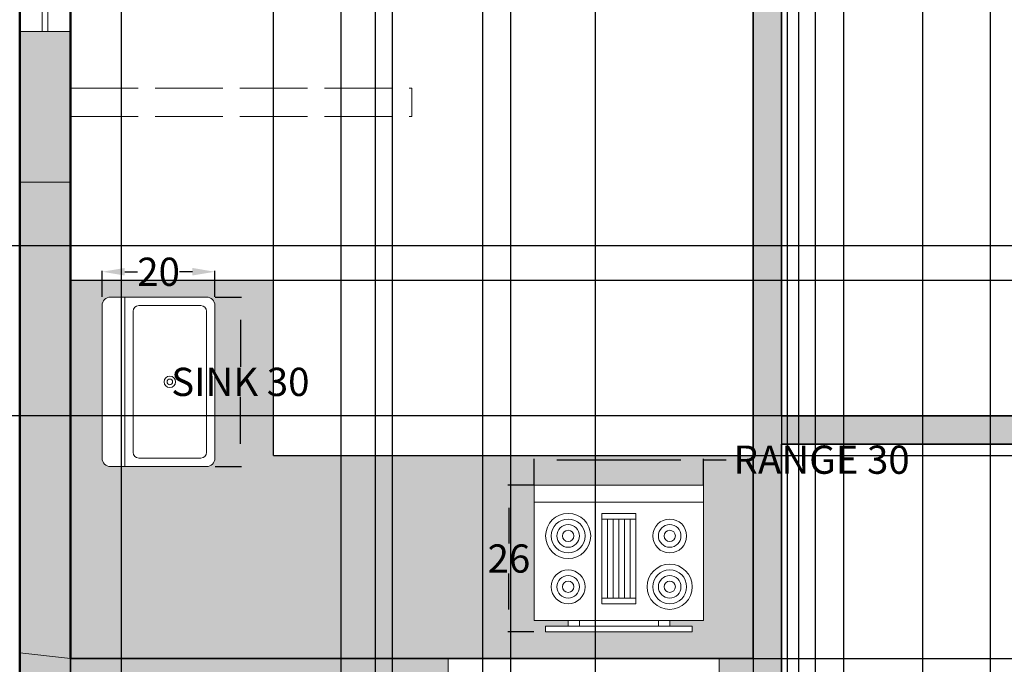
# Model space of a CAD drawing. Units: inches. Extents: x 882 to 1363, y 890 to 1847.
# Tile 3 of 9: x 983 to 1157, y 1106 to 1220. Entities that reach past the tile are written whole.
import ezdxf

# ---------------------------------------------------------------- set-up
doc = ezdxf.new("R2010")
doc.units = ezdxf.units.IN
doc.header["$MEASUREMENT"] = 0
doc.linetypes.add('ACAD_ISO02W100', pattern=[15, 12, -3])
for name, color, linetype, lineweight in [('A-ANNO-DIMS', 2, 'Continuous', 18), ('A-EQPM', 8, 'Continuous', 18), ('A-FLOR-CASE', 7, 'Continuous', 25), ('A-WALL-OVHD', 7, 'ACAD_ISO02W100', 18), ('A-WALL-PATT-BNDY', 7, 'Continuous', 13), ('inner wall', 50, 'Continuous', 35), ('outer wall', 40, 'Continuous', 50), ('sanitary', 231, 'Continuous', 18), ('windows', 226, 'Continuous', 18)]:
    doc.layers.add(name, color=color, linetype=linetype, lineweight=lineweight)
doc.layers.add('A-FLOR-CASE-PATT', color=15, linetype='Continuous', lineweight=13, true_color=0x9c4f2b)
doc.layers.add('A-WALL-PATT', color=251, linetype='Continuous', lineweight=13, true_color=0x636466)
doc.styles.get("Standard").update_dxf_attribs({"font": 'arial.ttf'})
doc.dimstyles.get("Standard").update_dxf_attribs({"dimtxt": 5, "dimasz": 4, "dimexe": 0.18, "dimexo": 0.0625, "dimgap": 0.09, "dimtad": 0, "dimtih": 1, "dimtoh": 1, "dimdec": 1, "dimzin": 0, "dimdsep": 46, "dimlunit": 3, "dimtxsty": 'Standard', "dimcen": 0.09, "dimadec": 0, "dimazin": 0, "dimtfac": 1, "dimtdec": 1, "dimtofl": 0, "dimtmove": 0, "dimatfit": 3, "dimfxl": 1, "dimtolj": 1, "dimtzin": 0, "dimarcsym": 0})

# ---------------------------------------------------------------- blocks, each defined once
blk = doc.blocks.new('Range-Oven - 30 in top')
for p, q in [((0, -3), (30, -3)), ((12, -6), (18, -6)), ((13, -20), (13, -6)), ((14, -6), (14, -20)), ((15, -20), (15, -6)), ((16, -6), (16, -20)), ((17, -20), (17, -6)), ((18, -20), (12, -20)), ((6, -24), (6, -25)), ((8, -25), (8, -24)), ((22, -25), (22, -24)), ((24, -24), (24, -25))]:
    blk.add_line(p, q)
for points in [[(0, -24), (0, 0), (30, 0), (30, -24)], [(12, -21), (12, -5), (18, -5), (18, -21)], [(2, -26), (2, -25), (28, -25), (28, -26)]]:
    blk.add_lwpolyline(points, close=True)
for centre, radius in [((6, -9), 4), ((6, -9), 3), ((24, -9), 3), ((6, -9), 2), ((6, -9), 1), ((24, -9), 2), ((24, -9), 1), ((6, -18), 3), ((24, -18), 4), ((24, -18), 3), ((6, -18), 2), ((6, -18), 1), ((24, -18), 2), ((24, -18), 1)]:
    blk.add_circle(centre, radius)
blk = doc.blocks.new('Sink-single - 30 in top')
blk.add_line((-15, -3.999996), (15, -3.999996))
for points in [[(-13.5, 0), (13.5, 0)], [(-15, -18.499996), (-15, -1.5)], [(15, -1.5), (15, -18.499996)], [(-13.5, -17.499996), (-13.5, -6.499996)], [(-12.5, -5.499996), (12.5, -5.499996)], [(13.5, -6.499996), (13.5, -17.499996)], [(12.5, -18.499996), (-12.5, -18.499996)], [(13.5, -19.999996), (-13.5, -19.999996)]]:
    blk.add_lwpolyline(points)
for radius in [1, 0.5]:
    blk.add_circle((0, -11.999996), radius)
for centre, radius, start, end in [((-13.5, -1.5), 1.5, 90, 180), ((13.5, -1.5), 1.5, 0, 90), ((-12.5, -6.499996), 1, 90, 180), ((12.5, -6.499996), 1, 0, 90), ((-13.5, -18.499996), 1.5, 180, 270), ((-12.5, -17.499996), 1, 180, 270), ((12.5, -17.499996), 1, 270, 0), ((13.5, -18.499996), 1.5, 270, 0)]:
    blk.add_arc(centre, radius, start, end)
blk = doc.blocks.new('WIN-48IN-9IN')
for p, q in [((4, 0), (4, 48)), ((5, 0), (5, 48))]:
    blk.add_line(p, q)
blk.add_lwpolyline([(0, 48), (9, 48), (9, 0), (0, 0)], close=True)
blk = doc.blocks.new('*D29')
at = {"layer": 'A-ANNO-DIMS', "color": 0, "lineweight": -2, "transparency": 16777216}
for p, q in [((1074.04, 1137.54), (1074.04, 1142.16)), ((1078.04, 1141.98), (1100.04, 1141.98)), ((1104.04, 1137.54), (1104.04, 1142.16)), ((1104.04, 1141.98), (1108.04, 1141.98))]:
    blk.add_line(p, q, dxfattribs=at)
at = {"layer": 'A-ANNO-DIMS', "color": 0, "transparency": 16777216}
for points in [[(1078.04, 1142.64), (1078.04, 1141.31), (1074.04, 1141.98)], [(1100.04, 1142.64), (1100.04, 1141.31), (1104.04, 1141.98)]]:
    blk.add_solid(points, dxfattribs=at)
at = {"layer": 'Defpoints', "color": 0, "transparency": 16777216}
for p in [(1104.04, 1141.98), (1074.04, 1137.48), (1104.04, 1137.48)]:
    blk.add_point(p, dxfattribs=at)
at = {"layer": 'A-ANNO-DIMS', "color": 0, "transparency": 16777216, "insert": (1124.96, 1141.98), "char_height": 5, "attachment_point": 5}
blk.add_mtext('\\A1;RANGE 30', dxfattribs=at)
blk = doc.blocks.new('*D30')
at = {"layer": 'A-ANNO-DIMS', "color": 0, "lineweight": -2, "transparency": 16777216}
for p, q in [((1073.98, 1137.48), (1069.36, 1137.48)), ((1069.54, 1133.48), (1069.54, 1127.12)), ((1069.54, 1115.48), (1069.54, 1121.83)), ((1073.98, 1111.48), (1069.36, 1111.48))]:
    blk.add_line(p, q, dxfattribs=at)
at = {"layer": 'A-ANNO-DIMS', "color": 0, "transparency": 16777216}
for points in [[(1068.87, 1133.48), (1070.2, 1133.48), (1069.54, 1137.48)], [(1068.87, 1115.48), (1070.2, 1115.48), (1069.54, 1111.48)]]:
    blk.add_solid(points, dxfattribs=at)
at = {"layer": 'Defpoints', "color": 0, "transparency": 16777216}
for p in [(1069.54, 1137.48), (1074.04, 1137.48), (1074.04, 1111.48)]:
    blk.add_point(p, dxfattribs=at)
at = {"layer": 'A-ANNO-DIMS', "color": 0, "transparency": 16777216, "insert": (1069.54, 1124.48), "char_height": 5, "attachment_point": 5}
blk.add_mtext('\\A1;26', dxfattribs=at)
blk = doc.blocks.new('*D31')
at = {"layer": 'A-ANNO-DIMS', "color": 0, "lineweight": -2, "transparency": 16777216}
for p, q in [((1017.51, 1170.76), (1022.13, 1170.76)), ((1021.95, 1166.76), (1021.95, 1158.44)), ((1021.95, 1144.76), (1021.95, 1153.09)), ((1017.51, 1140.76), (1022.13, 1140.76))]:
    blk.add_line(p, q, dxfattribs=at)
at = {"layer": 'A-ANNO-DIMS', "color": 0, "transparency": 16777216}
for points in [[(1021.28, 1166.76), (1022.61, 1166.76), (1021.95, 1170.76)], [(1021.28, 1144.76), (1022.61, 1144.76), (1021.95, 1140.76)]]:
    blk.add_solid(points, dxfattribs=at)
at = {"layer": 'Defpoints', "color": 0, "transparency": 16777216}
for p in [(1017.45, 1170.76), (1021.95, 1170.76), (1017.45, 1140.76)]:
    blk.add_point(p, dxfattribs=at)
at = {"layer": 'A-ANNO-DIMS', "color": 0, "transparency": 16777216, "insert": (1021.95, 1155.76), "char_height": 5, "attachment_point": 5}
blk.add_mtext('\\A1;SINK 30', dxfattribs=at)
blk = doc.blocks.new('*D32')
at = {"layer": 'A-ANNO-DIMS', "color": 0, "lineweight": -2, "transparency": 16777216}
for p, q in [((997.45, 1170.83), (997.45, 1175.44)), ((1001.45, 1175.26), (1003.74, 1175.26)), ((1013.45, 1175.26), (1011.15, 1175.26)), ((1017.45, 1170.83), (1017.45, 1175.44))]:
    blk.add_line(p, q, dxfattribs=at)
at = {"layer": 'A-ANNO-DIMS', "color": 0, "transparency": 16777216}
for points in [[(1001.45, 1175.93), (1001.45, 1174.6), (997.45, 1175.26)], [(1013.45, 1175.93), (1013.45, 1174.6), (1017.45, 1175.26)]]:
    blk.add_solid(points, dxfattribs=at)
at = {"layer": 'Defpoints', "color": 0, "transparency": 16777216}
for p in [(997.45, 1175.26), (997.45, 1170.76), (1017.45, 1170.76)]:
    blk.add_point(p, dxfattribs=at)
at = {"layer": 'A-ANNO-DIMS', "color": 0, "transparency": 16777216, "insert": (1007.45, 1175.26), "char_height": 5, "attachment_point": 5}
blk.add_mtext('\\A1;20', dxfattribs=at)
blk = doc.blocks.new('*D40')
at = {"layer": 'A-ANNO-DIMS', "color": 0, "lineweight": -2, "transparency": 16777216}
for p, q in [((991.84, 1758.69), (991.84, 893.37)), ((1064.84, 1758.69), (1064.84, 893.37)), ((995.84, 893.55), (1024.69, 893.55)), ((1060.84, 893.55), (1031.99, 893.55))]:
    blk.add_line(p, q, dxfattribs=at)
at = {"layer": 'A-ANNO-DIMS', "color": 0, "transparency": 16777216}
for points in [[(995.84, 894.21), (995.84, 892.88), (991.84, 893.55)], [(1060.84, 894.21), (1060.84, 892.88), (1064.84, 893.55)]]:
    blk.add_solid(points, dxfattribs=at)
at = {"layer": 'Defpoints', "color": 0, "transparency": 16777216}
for p in [(991.84, 1758.75), (1064.84, 1758.75), (1064.84, 893.55)]:
    blk.add_point(p, dxfattribs=at)
at = {"layer": 'A-ANNO-DIMS', "color": 0, "transparency": 16777216, "insert": (1028.34, 893.55), "char_height": 5, "attachment_point": 5}
blk.add_mtext('\\A1;73', dxfattribs=at)
blk = doc.blocks.new('*D41')
at = {"layer": 'A-ANNO-DIMS', "color": 0, "lineweight": -2, "transparency": 16777216}
for p, q in [((1069.84, 1758.69), (1069.84, 893.37)), ((1154.84, 1758.69), (1154.84, 893.37)), ((1073.84, 893.55), (1108.65, 893.55)), ((1150.84, 893.55), (1116.03, 893.55))]:
    blk.add_line(p, q, dxfattribs=at)
at = {"layer": 'A-ANNO-DIMS', "color": 0, "transparency": 16777216}
for points in [[(1073.84, 894.21), (1073.84, 892.88), (1069.84, 893.55)], [(1150.84, 894.21), (1150.84, 892.88), (1154.84, 893.55)]]:
    blk.add_solid(points, dxfattribs=at)
at = {"layer": 'Defpoints', "color": 0, "transparency": 16777216}
for p in [(1069.84, 1758.75), (1154.84, 1758.75), (1154.84, 893.55)]:
    blk.add_point(p, dxfattribs=at)
at = {"layer": 'A-ANNO-DIMS', "color": 0, "transparency": 16777216, "insert": (1112.34, 893.55), "char_height": 5, "attachment_point": 5}
blk.add_mtext('\\A1;85', dxfattribs=at)
blk = doc.blocks.new('*D47')
at = {"layer": 'A-ANNO-DIMS', "color": 0, "lineweight": -2, "transparency": 16777216}
for p, q in [((1123.84, 1567.69), (1123.84, 893.37)), ((1128.84, 1567.69), (1128.84, 893.37)), ((1119.84, 893.55), (1115.84, 893.55)), ((1132.84, 893.55), (1136.84, 893.55))]:
    blk.add_line(p, q, dxfattribs=at)
at = {"layer": 'A-ANNO-DIMS', "color": 0, "transparency": 16777216}
for points in [[(1119.84, 894.21), (1119.84, 892.88), (1123.84, 893.55)], [(1132.84, 894.21), (1132.84, 892.88), (1128.84, 893.55)]]:
    blk.add_solid(points, dxfattribs=at)
at = {"layer": 'Defpoints', "color": 0, "transparency": 16777216}
for p in [(1123.84, 1567.75), (1128.84, 1567.75), (1128.84, 893.55)]:
    blk.add_point(p, dxfattribs=at)
at = {"layer": 'A-ANNO-DIMS', "color": 0, "transparency": 16777216, "insert": (1126.34, 893.55), "char_height": 5, "attachment_point": 5}
blk.add_mtext('\\A1;5', dxfattribs=at)
blk = doc.blocks.new('*D48')
at = {"layer": 'A-ANNO-DIMS', "color": 0, "lineweight": -2, "transparency": 16777216}
for p, q in [((1084.84, 1562.69), (1084.84, 893.37)), ((1120.84, 1562.69), (1120.84, 893.37)), ((1088.84, 893.55), (1099.17, 893.55)), ((1116.84, 893.55), (1106.51, 893.55))]:
    blk.add_line(p, q, dxfattribs=at)
at = {"layer": 'A-ANNO-DIMS', "color": 0, "transparency": 16777216}
for points in [[(1088.84, 894.21), (1088.84, 892.88), (1084.84, 893.55)], [(1116.84, 894.21), (1116.84, 892.88), (1120.84, 893.55)]]:
    blk.add_solid(points, dxfattribs=at)
at = {"layer": 'Defpoints', "color": 0, "transparency": 16777216}
for p in [(1084.84, 1562.75), (1120.84, 1562.75), (1120.84, 893.55)]:
    blk.add_point(p, dxfattribs=at)
at = {"layer": 'A-ANNO-DIMS', "color": 0, "transparency": 16777216, "insert": (1102.84, 893.55), "char_height": 5, "attachment_point": 5}
blk.add_mtext('\\A1;36', dxfattribs=at)
blk = doc.blocks.new('*D51')
at = {"layer": 'A-ANNO-DIMS', "color": 0, "lineweight": -2, "transparency": 16777216}
for p, q in [((982.84, 1767.69), (982.84, 893.37)), ((1000.84, 1767.69), (1000.84, 893.37)), ((986.84, 893.55), (996.84, 893.55)), ((1000.84, 893.55), (1004.84, 893.55))]:
    blk.add_line(p, q, dxfattribs=at)
at = {"layer": 'A-ANNO-DIMS', "color": 0, "transparency": 16777216}
for points in [[(986.84, 894.21), (986.84, 892.88), (982.84, 893.55)], [(996.84, 894.21), (996.84, 892.88), (1000.84, 893.55)]]:
    blk.add_solid(points, dxfattribs=at)
at = {"layer": 'Defpoints', "color": 0, "transparency": 16777216}
for p in [(982.84, 1767.75), (1000.84, 1767.75), (1000.84, 893.55)]:
    blk.add_point(p, dxfattribs=at)
at = {"layer": 'A-ANNO-DIMS', "color": 0, "transparency": 16777216, "insert": (1015.08, 893.55), "char_height": 5, "attachment_point": 5}
blk.add_mtext('\\A1;18.006', dxfattribs=at)
blk = doc.blocks.new('*D52')
at = {"layer": 'A-ANNO-DIMS', "color": 0, "lineweight": -2, "transparency": 16777216}
for p, q in [((1048.84, 1767.69), (1048.84, 893.37)), ((1118.86, 1767.69), (1118.86, 893.37)), ((1052.84, 893.55), (1075.83, 893.55)), ((1114.86, 893.55), (1091.87, 893.55))]:
    blk.add_line(p, q, dxfattribs=at)
at = {"layer": 'A-ANNO-DIMS', "color": 0, "transparency": 16777216}
for points in [[(1052.84, 894.21), (1052.84, 892.88), (1048.84, 893.55)], [(1114.86, 894.21), (1114.86, 892.88), (1118.86, 893.55)]]:
    blk.add_solid(points, dxfattribs=at)
at = {"layer": 'Defpoints', "color": 0, "transparency": 16777216}
for p in [(1048.84, 1767.75), (1118.86, 1767.75), (1118.86, 893.55)]:
    blk.add_point(p, dxfattribs=at)
at = {"layer": 'A-ANNO-DIMS', "color": 0, "transparency": 16777216, "insert": (1083.85, 893.55), "char_height": 5, "attachment_point": 5}
blk.add_mtext('\\A1;70.01', dxfattribs=at)
blk = doc.blocks.new('*D53')
at = {"layer": 'A-ANNO-DIMS', "color": 0, "lineweight": -2, "transparency": 16777216}
for p, q in [((1142.86, 1767.69), (1142.86, 893.37)), ((1171.41, 1767.69), (1171.41, 893.37)), ((1138.86, 893.55), (1134.86, 893.55)), ((1175.41, 893.55), (1179.41, 893.55))]:
    blk.add_line(p, q, dxfattribs=at)
at = {"layer": 'A-ANNO-DIMS', "color": 0, "transparency": 16777216}
for points in [[(1138.86, 894.21), (1138.86, 892.88), (1142.86, 893.55)], [(1175.41, 894.21), (1175.41, 892.88), (1171.41, 893.55)]]:
    blk.add_solid(points, dxfattribs=at)
at = {"layer": 'Defpoints', "color": 0, "transparency": 16777216}
for p in [(1142.86, 1767.75), (1171.41, 1767.75), (1171.41, 893.55)]:
    blk.add_point(p, dxfattribs=at)
at = {"layer": 'A-ANNO-DIMS', "color": 0, "transparency": 16777216, "insert": (1157.14, 893.55), "char_height": 5, "attachment_point": 5}
blk.add_mtext('\\A1;28.554', dxfattribs=at)
blk = doc.blocks.new('*D61')
at = {"layer": 'A-ANNO-DIMS', "color": 0, "lineweight": -2, "transparency": 16777216}
for p, q in [((991.84, 1348.69), (991.84, 893.37)), ((1128.84, 1348.69), (1128.84, 893.37)), ((995.84, 893.55), (1054.96, 893.55)), ((1124.84, 893.55), (1065.72, 893.55))]:
    blk.add_line(p, q, dxfattribs=at)
at = {"layer": 'A-ANNO-DIMS', "color": 0, "transparency": 16777216}
for points in [[(995.84, 894.21), (995.84, 892.88), (991.84, 893.55)], [(1124.84, 894.21), (1124.84, 892.88), (1128.84, 893.55)]]:
    blk.add_solid(points, dxfattribs=at)
at = {"layer": 'Defpoints', "color": 0, "transparency": 16777216}
for p in [(991.84, 1348.75), (1128.84, 1348.75), (1128.84, 893.55)]:
    blk.add_point(p, dxfattribs=at)
at = {"layer": 'A-ANNO-DIMS', "color": 0, "transparency": 16777216, "insert": (1060.34, 893.55), "char_height": 5, "attachment_point": 5}
blk.add_mtext('\\A1;137', dxfattribs=at)
blk = doc.blocks.new('*D62')
at = {"layer": 'A-ANNO-DIMS', "color": 0, "lineweight": -2, "transparency": 16777216}
for p, q in [((991.9, 1348.75), (1353.22, 1348.75)), ((1353.04, 1344.75), (1353.04, 1230.35)), ((1353.04, 1110.75), (1353.04, 1225.15)), ((991.9, 1106.75), (1353.22, 1106.75))]:
    blk.add_line(p, q, dxfattribs=at)
at = {"layer": 'A-ANNO-DIMS', "color": 0, "transparency": 16777216}
for points in [[(1352.38, 1344.75), (1353.71, 1344.75), (1353.04, 1348.75)], [(1352.38, 1110.75), (1353.71, 1110.75), (1353.04, 1106.75)]]:
    blk.add_solid(points, dxfattribs=at)
at = {"layer": 'Defpoints', "color": 0, "transparency": 16777216}
for p in [(991.84, 1348.75), (991.84, 1106.75), (1353.04, 1106.75)]:
    blk.add_point(p, dxfattribs=at)
at = {"layer": 'A-ANNO-DIMS', "color": 0, "transparency": 16777216, "insert": (1353.04, 1227.75), "char_height": 5, "attachment_point": 5}
blk.add_mtext('\\A1;242', dxfattribs=at)
blk = doc.blocks.new('*D63')
at = {"layer": 'A-ANNO-DIMS', "color": 0, "lineweight": -2, "transparency": 16777216}
for p, q in [((991.84, 1106.69), (991.84, 893.37)), ((1112.84, 1106.69), (1112.84, 893.37)), ((995.84, 893.55), (1047.44, 893.55)), ((1108.84, 893.55), (1057.23, 893.55))]:
    blk.add_line(p, q, dxfattribs=at)
at = {"layer": 'A-ANNO-DIMS', "color": 0, "transparency": 16777216}
for points in [[(995.84, 894.21), (995.84, 892.88), (991.84, 893.55)], [(1108.84, 894.21), (1108.84, 892.88), (1112.84, 893.55)]]:
    blk.add_solid(points, dxfattribs=at)
at = {"layer": 'Defpoints', "color": 0, "transparency": 16777216}
for p in [(991.84, 1106.75), (1112.84, 1106.75), (1112.84, 893.55)]:
    blk.add_point(p, dxfattribs=at)
at = {"layer": 'A-ANNO-DIMS', "color": 0, "transparency": 16777216, "insert": (1052.34, 893.55), "char_height": 5, "attachment_point": 5}
blk.add_mtext('\\A1;121', dxfattribs=at)
blk = doc.blocks.new('*D64')
at = {"layer": 'A-ANNO-DIMS', "color": 0, "lineweight": -2, "transparency": 16777216}
for p, q in [((1117.84, 1269.69), (1117.84, 893.37)), ((1243.84, 1269.69), (1243.84, 893.37)), ((1121.84, 893.55), (1175.46, 893.55)), ((1239.84, 893.55), (1186.22, 893.55))]:
    blk.add_line(p, q, dxfattribs=at)
at = {"layer": 'A-ANNO-DIMS', "color": 0, "transparency": 16777216}
for points in [[(1121.84, 894.21), (1121.84, 892.88), (1117.84, 893.55)], [(1239.84, 894.21), (1239.84, 892.88), (1243.84, 893.55)]]:
    blk.add_solid(points, dxfattribs=at)
at = {"layer": 'Defpoints', "color": 0, "transparency": 16777216}
for p in [(1117.84, 1269.75), (1243.84, 1269.75), (1243.84, 893.55)]:
    blk.add_point(p, dxfattribs=at)
at = {"layer": 'A-ANNO-DIMS', "color": 0, "transparency": 16777216, "insert": (1180.84, 893.55), "char_height": 5, "attachment_point": 5}
blk.add_mtext('\\A1;126', dxfattribs=at)
blk = doc.blocks.new('*D65')
at = {"layer": 'A-ANNO-DIMS', "color": 0, "lineweight": -2, "transparency": 16777216}
for p, q in [((1117.9, 1269.75), (1353.22, 1269.75)), ((1353.04, 1265.75), (1353.04, 1212.39)), ((1353.04, 1153.75), (1353.04, 1207.11)), ((1117.9, 1149.75), (1353.22, 1149.75))]:
    blk.add_line(p, q, dxfattribs=at)
at = {"layer": 'A-ANNO-DIMS', "color": 0, "transparency": 16777216}
for points in [[(1352.38, 1265.75), (1353.71, 1265.75), (1353.04, 1269.75)], [(1352.38, 1153.75), (1353.71, 1153.75), (1353.04, 1149.75)]]:
    blk.add_solid(points, dxfattribs=at)
at = {"layer": 'Defpoints', "color": 0, "transparency": 16777216}
for p in [(1117.84, 1269.75), (1353.04, 1269.75), (1117.84, 1149.75)]:
    blk.add_point(p, dxfattribs=at)
at = {"layer": 'A-ANNO-DIMS', "color": 0, "transparency": 16777216, "insert": (1353.04, 1209.75), "char_height": 5, "attachment_point": 5}
blk.add_mtext('\\A1;120', dxfattribs=at)
blk = doc.blocks.new('*D68')
at = {"layer": 'A-ANNO-DIMS', "color": 0, "lineweight": -2, "transparency": 16777216}
for p, q in [((1027.84, 1142.81), (1027.84, 1844.13)), ((1031.84, 1843.95), (1066.65, 1843.95)), ((1108.84, 1843.95), (1074.03, 1843.95)), ((1112.84, 1142.81), (1112.84, 1844.13))]:
    blk.add_line(p, q, dxfattribs=at)
at = {"layer": 'A-ANNO-DIMS', "color": 0, "transparency": 16777216}
for points in [[(1031.84, 1844.62), (1031.84, 1843.29), (1027.84, 1843.95)], [(1108.84, 1844.62), (1108.84, 1843.29), (1112.84, 1843.95)]]:
    blk.add_solid(points, dxfattribs=at)
at = {"layer": 'Defpoints', "color": 0, "transparency": 16777216}
for p in [(1112.84, 1843.95), (1027.84, 1142.75), (1112.84, 1142.75)]:
    blk.add_point(p, dxfattribs=at)
at = {"layer": 'A-ANNO-DIMS', "color": 0, "transparency": 16777216, "insert": (1070.34, 1843.95), "char_height": 5, "attachment_point": 5}
blk.add_mtext('\\A1;85', dxfattribs=at)
blk = doc.blocks.new('*D69')
at = {"layer": 'A-ANNO-DIMS', "color": 0, "lineweight": -2, "transparency": 16777216}
for p, q in [((1027.9, 1173.75), (1353.22, 1173.75)), ((1353.04, 1169.75), (1353.04, 1160.89)), ((1353.04, 1146.75), (1353.04, 1155.6)), ((1027.9, 1142.75), (1353.22, 1142.75))]:
    blk.add_line(p, q, dxfattribs=at)
at = {"layer": 'A-ANNO-DIMS', "color": 0, "transparency": 16777216}
for points in [[(1352.38, 1169.75), (1353.71, 1169.75), (1353.04, 1173.75)], [(1352.38, 1146.75), (1353.71, 1146.75), (1353.04, 1142.75)]]:
    blk.add_solid(points, dxfattribs=at)
at = {"layer": 'Defpoints', "color": 0, "transparency": 16777216}
for p in [(1027.84, 1173.75), (1353.04, 1173.75), (1027.84, 1142.75)]:
    blk.add_point(p, dxfattribs=at)
at = {"layer": 'A-ANNO-DIMS', "color": 0, "transparency": 16777216, "insert": (1353.04, 1158.25), "char_height": 5, "attachment_point": 5}
blk.add_mtext('\\A1;31', dxfattribs=at)
blk = doc.blocks.new('*D70')
at = {"layer": 'A-ANNO-DIMS', "color": 0, "lineweight": -2, "transparency": 16777216}
for p, q in [((1027.9, 1142.75), (1353.22, 1142.75)), ((1353.04, 1138.75), (1353.04, 1127.39)), ((1353.04, 1110.75), (1353.04, 1122.1)), ((991.9, 1106.75), (1353.22, 1106.75))]:
    blk.add_line(p, q, dxfattribs=at)
at = {"layer": 'A-ANNO-DIMS', "color": 0, "transparency": 16777216}
for points in [[(1352.38, 1138.75), (1353.71, 1138.75), (1353.04, 1142.75)], [(1352.38, 1110.75), (1353.71, 1110.75), (1353.04, 1106.75)]]:
    blk.add_solid(points, dxfattribs=at)
at = {"layer": 'Defpoints', "color": 0, "transparency": 16777216}
for p in [(1027.84, 1142.75), (991.84, 1106.75), (1353.04, 1106.75)]:
    blk.add_point(p, dxfattribs=at)
at = {"layer": 'A-ANNO-DIMS', "color": 0, "transparency": 16777216, "insert": (1353.04, 1124.75), "char_height": 5, "attachment_point": 5}
blk.add_mtext('\\A1;36', dxfattribs=at)
blk = doc.blocks.new('*D71')
at = {"layer": 'A-ANNO-DIMS', "color": 0, "lineweight": -2, "transparency": 16777216}
for p, q in [((1243.78, 1179.86), (906.46, 1179.86)), ((906.64, 1175.86), (906.64, 1167.45)), ((906.64, 1153.75), (906.64, 1162.16)), ((1243.78, 1149.75), (906.46, 1149.75))]:
    blk.add_line(p, q, dxfattribs=at)
at = {"layer": 'A-ANNO-DIMS', "color": 0, "transparency": 16777216}
for points in [[(905.97, 1175.86), (907.3, 1175.86), (906.64, 1179.86)], [(905.97, 1153.75), (907.3, 1153.75), (906.64, 1149.75)]]:
    blk.add_solid(points, dxfattribs=at)
at = {"layer": 'Defpoints', "color": 0, "transparency": 16777216}
for p in [(906.64, 1179.86), (1243.84, 1179.86), (1243.84, 1149.75)]:
    blk.add_point(p, dxfattribs=at)
at = {"layer": 'A-ANNO-DIMS', "color": 0, "transparency": 16777216, "insert": (906.64, 1164.8), "char_height": 5, "attachment_point": 5}
blk.add_mtext('\\A1;30.107', dxfattribs=at)
blk = doc.blocks.new('*D74')
at = {"layer": 'A-ANNO-DIMS', "color": 0, "lineweight": -2, "transparency": 16777216}
for p, q in [((991.84, 1002.81), (991.84, 1844.13)), ((995.84, 1843.95), (1012.06, 1843.95)), ((1035.84, 1843.95), (1019.62, 1843.95)), ((1039.84, 1002.81), (1039.84, 1844.13))]:
    blk.add_line(p, q, dxfattribs=at)
at = {"layer": 'A-ANNO-DIMS', "color": 0, "transparency": 16777216}
for points in [[(995.84, 1844.62), (995.84, 1843.29), (991.84, 1843.95)], [(1035.84, 1844.62), (1035.84, 1843.29), (1039.84, 1843.95)]]:
    blk.add_solid(points, dxfattribs=at)
at = {"layer": 'Defpoints', "color": 0, "transparency": 16777216}
for p in [(1039.84, 1843.95), (991.84, 1002.75), (1039.84, 1002.75)]:
    blk.add_point(p, dxfattribs=at)
at = {"layer": 'A-ANNO-DIMS', "color": 0, "transparency": 16777216, "insert": (1015.84, 1843.95), "char_height": 5, "attachment_point": 5}
blk.add_mtext('\\A1;48', dxfattribs=at)
blk = doc.blocks.new('*D77')
at = {"layer": 'A-ANNO-DIMS', "color": 0, "lineweight": -2, "transparency": 16777216}
for p, q in [((1117.9, 1144.75), (1353.22, 1144.75)), ((1353.04, 1140.75), (1353.04, 1125.89)), ((1353.04, 1105.75), (1353.04, 1120.6)), ((1117.9, 1101.75), (1353.22, 1101.75))]:
    blk.add_line(p, q, dxfattribs=at)
at = {"layer": 'A-ANNO-DIMS', "color": 0, "transparency": 16777216}
for points in [[(1352.38, 1140.75), (1353.71, 1140.75), (1353.04, 1144.75)], [(1352.38, 1105.75), (1353.71, 1105.75), (1353.04, 1101.75)]]:
    blk.add_solid(points, dxfattribs=at)
at = {"layer": 'Defpoints', "color": 0, "transparency": 16777216}
for p in [(1117.84, 1144.75), (1353.04, 1144.75), (1117.84, 1101.75)]:
    blk.add_point(p, dxfattribs=at)
at = {"layer": 'A-ANNO-DIMS', "color": 0, "transparency": 16777216, "insert": (1353.04, 1123.25), "char_height": 5, "attachment_point": 5}
blk.add_mtext('\\A1;43', dxfattribs=at)
blk = doc.blocks.new('*D85')
at = {"layer": 'A-ANNO-DIMS', "color": 0, "lineweight": -2, "transparency": 16777216}
for p, q in [((1045.84, 1562.69), (1045.84, 893.37)), ((1084.84, 1562.69), (1084.84, 893.37)), ((1049.84, 893.55), (1061.66, 893.55)), ((1080.84, 893.55), (1069.01, 893.55))]:
    blk.add_line(p, q, dxfattribs=at)
at = {"layer": 'A-ANNO-DIMS', "color": 0, "transparency": 16777216}
for points in [[(1049.84, 894.21), (1049.84, 892.88), (1045.84, 893.55)], [(1080.84, 894.21), (1080.84, 892.88), (1084.84, 893.55)]]:
    blk.add_solid(points, dxfattribs=at)
at = {"layer": 'Defpoints', "color": 0, "transparency": 16777216}
for p in [(1045.84, 1562.75), (1084.84, 1562.75), (1084.84, 893.55)]:
    blk.add_point(p, dxfattribs=at)
at = {"layer": 'A-ANNO-DIMS', "color": 0, "transparency": 16777216, "insert": (1065.34, 893.55), "char_height": 5, "attachment_point": 5}
blk.add_mtext('\\A1;39', dxfattribs=at)
blk = doc.blocks.new('*D88')
at = {"layer": 'A-ANNO-DIMS', "color": 0, "lineweight": -2, "transparency": 16777216}
for p, q in [((1128.84, 1567.69), (1128.84, 893.37)), ((1211.84, 1562.69), (1211.84, 893.37)), ((1132.84, 893.55), (1166.66, 893.55)), ((1207.84, 893.55), (1174.01, 893.55))]:
    blk.add_line(p, q, dxfattribs=at)
at = {"layer": 'A-ANNO-DIMS', "color": 0, "transparency": 16777216}
for points in [[(1132.84, 894.21), (1132.84, 892.88), (1128.84, 893.55)], [(1207.84, 894.21), (1207.84, 892.88), (1211.84, 893.55)]]:
    blk.add_solid(points, dxfattribs=at)
at = {"layer": 'Defpoints', "color": 0, "transparency": 16777216}
for p in [(1128.84, 1567.75), (1211.84, 1562.75), (1211.84, 893.55)]:
    blk.add_point(p, dxfattribs=at)
at = {"layer": 'A-ANNO-DIMS', "color": 0, "transparency": 16777216, "insert": (1170.34, 893.55), "char_height": 5, "attachment_point": 5}
blk.add_mtext('\\A1;83', dxfattribs=at)
blk = doc.blocks.new('*D89')
at = {"layer": 'A-ANNO-DIMS', "color": 0, "lineweight": -2, "transparency": 16777216}
for p, q in [((991.84, 1473.69), (991.84, 893.37)), ((1084.84, 1473.69), (1084.84, 893.37)), ((995.84, 893.55), (1034.67, 893.55)), ((1080.84, 893.55), (1042.01, 893.55))]:
    blk.add_line(p, q, dxfattribs=at)
at = {"layer": 'A-ANNO-DIMS', "color": 0, "transparency": 16777216}
for points in [[(995.84, 894.21), (995.84, 892.88), (991.84, 893.55)], [(1080.84, 894.21), (1080.84, 892.88), (1084.84, 893.55)]]:
    blk.add_solid(points, dxfattribs=at)
at = {"layer": 'Defpoints', "color": 0, "transparency": 16777216}
for p in [(991.84, 1473.75), (1084.84, 1473.75), (1084.84, 893.55)]:
    blk.add_point(p, dxfattribs=at)
at = {"layer": 'A-ANNO-DIMS', "color": 0, "transparency": 16777216, "insert": (1038.34, 893.55), "char_height": 5, "attachment_point": 5}
blk.add_mtext('\\A1;93', dxfattribs=at)

msp = doc.modelspace()

# ---------------------------------------------------------------- hatches: boundary and pattern name
at = {"layer": 'A-FLOR-CASE-PATT'}
h = msp.add_hatch(color=256, dxfattribs=at)
h.dxf.hatch_style = 1
h.paths.add_polyline_path([(1112.8388, 1142.7495), (1027.8388, 1142.7495), (1027.8388, 1173.7495), (991.8388, 1173.7495), (991.8388, 1106.7495), (1112.8388, 1106.7495)])
h.paths.add_polyline_path([(1074.0381, 1137.4754), (1104.0381, 1137.4754), (1104.0381, 1113.4754), (1098.0381, 1113.4754), (1098.0381, 1112.4754), (1102.0381, 1112.4754), (1102.0381, 1111.4754), (1076.0381, 1111.4754), (1076.0381, 1112.4754), (1080.0381, 1112.4754), (1080.0381, 1113.4754), (1074.0381, 1113.4754)], flags=16)
h.paths.add_polyline_path([(1076.0381, 1128.4754, -1), (1084.0381, 1128.4754, -1)], flags=0)
h.paths.add_polyline_path([(1077.0381, 1128.4754, -1), (1083.0381, 1128.4754, -1)], flags=0)
h.paths.add_polyline_path([(1083.0381, 1119.4754, -1), (1077.0381, 1119.4754, -1)], flags=0)
h.paths.add_polyline_path([(1082.0381, 1128.4754, -1), (1078.0381, 1128.4754, -1)], flags=0)
h.paths.add_polyline_path([(1082.0381, 1119.4754, -1), (1078.0381, 1119.4754, -1)], flags=0)
h.paths.add_polyline_path([(1081.0381, 1128.4754, -1), (1079.0381, 1128.4754, -1)], flags=0)
h.paths.add_polyline_path([(1081.0381, 1119.4754, -1), (1079.0381, 1119.4754, -1)], flags=0)
h.paths.add_polyline_path([(1015.946, 1140.7644), (998.946, 1140.7644, -0.41421356), (997.446, 1142.2644), (997.446, 1169.2644, -0.41421356), (998.946, 1170.7644), (1015.946, 1170.7644, -0.41421356), (1017.446, 1169.2644), (1017.446, 1142.2644, -0.41421356)], flags=16)
h.paths.add_polyline_path([(1014.946, 1142.2644), (1003.946, 1142.2644, -0.41421356), (1002.946, 1143.2644), (1002.946, 1168.2644, -0.41421356), (1003.946, 1169.2644), (1014.946, 1169.2644, -0.41421356), (1015.946, 1168.2644), (1015.946, 1143.2644, -0.41421356)], flags=0)
h.paths.add_polyline_path([(1086.0381, 1132.4754), (1092.0381, 1132.4754), (1092.0381, 1116.4754), (1086.0381, 1116.4754)], flags=0)
h.paths.add_polyline_path([(1091.0381, 1131.4754), (1091.0381, 1117.4754), (1087.0381, 1117.4754), (1087.0381, 1131.4754)], flags=0)
h.paths.add_polyline_path([(1102.0381, 1119.4754, -1), (1094.0381, 1119.4754, -1)], flags=0)
h.paths.add_polyline_path([(1101.0381, 1128.4754, -1), (1095.0381, 1128.4754, -1)], flags=0)
h.paths.add_polyline_path([(1101.0381, 1119.4754, -1), (1095.0381, 1119.4754, -1)], flags=0)
h.paths.add_polyline_path([(1008.446, 1155.7644, -1), (1010.446, 1155.7644, -1)], flags=0)
h.paths.add_polyline_path([(1100.0381, 1128.4754, -1), (1096.0381, 1128.4754, -1)], flags=0)
h.paths.add_polyline_path([(1100.0381, 1119.4754, -1), (1096.0381, 1119.4754, -1)], flags=0)
h.paths.add_polyline_path([(1008.946, 1155.7644, -1), (1009.946, 1155.7644, -1)], flags=0)
h.paths.add_polyline_path([(1099.0381, 1128.4754, -1), (1097.0381, 1128.4754, -1)], flags=0)
h.paths.add_polyline_path([(1099.0381, 1119.4754, -1), (1097.0381, 1119.4754, -1)], flags=0)
at = {"layer": 'A-WALL-PATT'}
h = msp.add_hatch(color=256, dxfattribs=at)
h.dxf.hatch_style = 1
h.paths.add_polyline_path([(1050.8388, 1481.7495), (1050.8388, 1478.7495), (1084.8388, 1478.7495), (1084.8388, 1473.7495), (991.8388, 1473.7495), (991.8388, 1361.0778), (982.8388, 1361.0778), (982.8388, 1556.1531), (991.8388, 1556.1531), (991.8388, 1478.7495), (1045.8388, 1478.7495), (1045.8388, 1481.7479), (1045.4161, 1481.7477), (1030.9055, 1506.8563), (1032.004, 1507.4911), (1046.5146, 1482.3825), (1045.4161, 1481.7477), (1045.8388, 1481.7479), (1045.8388, 1481.7495)])
h.paths.add_polyline_path([(1128.8388, 1478.7495), (1120.8388, 1478.7495), (1120.8388, 1473.7495), (1123.8388, 1473.7495), (1123.8388, 1353.7495), (991.8388, 1353.7495), (991.8388, 1361.0778), (982.8388, 1361.0778), (982.8388, 1337.3333), (991.8388, 1337.3333), (991.8388, 1348.7495), (1128.8388, 1348.7495)])
h.paths.add_polyline_path([(1118.8585, 1767.7495), (1048.8447, 1767.7495), (1048.8447, 1758.7495), (1064.8388, 1758.7495), (1069.8388, 1758.7495), (1118.8585, 1758.7495)])
h.paths.add_polyline_path([(1171.4129, 1767.7495), (1142.8585, 1767.7495), (1142.8585, 1758.7495), (1154.8388, 1758.7495), (1154.8388, 1710.7495), (1069.8388, 1710.7495), (1069.8388, 1713.7495), (1064.8388, 1713.7495), (1064.8388, 1705.7495), (1123.8388, 1705.7495), (1123.8388, 1567.7495), (1120.8388, 1567.7495), (1120.8388, 1562.7495), (1123.8388, 1562.7495), (1211.8388, 1562.7495), (1211.8388, 1567.7495), (1128.8388, 1567.7495), (1128.8388, 1705.7495), (1211.8388, 1705.7495), (1211.8388, 1710.7495), (1159.8388, 1710.7495), (1159.8388, 1758.7495), (1171.4129, 1758.7495)])
h.paths.add_polyline_path([(1252.8388, 1767.7495), (1195.4129, 1767.7495), (1195.4129, 1758.7495), (1243.8388, 1758.7495), (1243.8388, 1710.7495), (1240.8388, 1710.7495), (1240.8388, 1706.4648), (1240.8388, 1705.7495), (1243.8388, 1705.7495), (1243.8388, 1673.1735), (1252.8388, 1673.1735)])
h.paths.add_polyline_path([(1252.8388, 1625.1735), (1243.8388, 1625.1735), (1243.8388, 1567.7495), (1240.8388, 1567.7495), (1240.8388, 1562.7495), (1243.8388, 1562.7495), (1243.8388, 1546.029), (1252.8388, 1546.029)])
h.paths.add_polyline_path([(1252.8388, 1498.029), (1243.8388, 1498.029), (1243.8388, 1391.1399), (1252.8388, 1391.1399)])
h.paths.add_polyline_path([(1252.8388, 1179.8561), (1243.8388, 1179.8561), (1243.8388, 1149.7495), (1219.8388, 1149.7495), (1219.8388, 1145.3111), (1219.8388, 1144.7495), (1252.8388, 1144.7495)])
h.paths.add_polyline_path([(1252.8388, 1277.7495), (1243.8388, 1277.7495), (1243.8388, 1274.7495), (1219.8388, 1274.7495), (1219.8388, 1269.7495), (1243.8388, 1269.7495), (1243.8388, 1227.8561), (1252.8388, 1227.8561)])
h.paths.add_polyline_path([(1252.8388, 1343.1399), (1243.8388, 1343.1399), (1243.8388, 1313.7495), (1248.3388, 1313.7495), (1252.8388, 1313.7495)])
h.paths.add_polyline_path([(1146.8388, 1274.7495), (1112.8388, 1274.7495), (1112.8388, 1106.7495), (1106.7761, 1106.7495), (1106.7761, 1101.7495), (1117.8388, 1101.7495), (1117.8388, 1144.7495), (1159.8388, 1144.7495), (1159.8388, 1149.7495), (1117.8388, 1149.7495), (1117.8388, 1269.7495), (1146.8388, 1269.7495)])
h = msp.add_hatch(color=256, dxfattribs=at)
h.dxf.hatch_style = 1
h.paths.add_polyline_path([(1000.8447, 1767.7495), (993.3979, 1767.7495), (991.8388, 1758.7495), (1000.8447, 1758.7495)])
h.paths.add_polyline_path([(991.8388, 1654.8981), (982.8388, 1654.3544), (982.8388, 1595.0521), (991.8388, 1594.8981)])
h.paths.add_polyline_path([(991.8388, 1594.8981), (982.8388, 1595.0521), (982.8388, 1559.7196), (991.8388, 1562.7495), (991.8388, 1567.7495)])
h.paths.add_polyline_path([(991.8388, 1562.7495), (982.8388, 1559.7196), (982.8388, 1556.1531), (991.8388, 1556.1531)])
h.paths.add_polyline_path([(991.8388, 1289.3333), (982.8388, 1289.3333), (982.8388, 1265.8272), (991.8388, 1265.8272)])
h.paths.add_polyline_path([(1058.7761, 1106.7495), (991.8388, 1106.7495), (982.8388, 1107.8066), (982.8388, 1101.3439), (991.8388, 1101.7495), (1058.7761, 1101.7495)])
h = msp.add_hatch(color=256, dxfattribs=at)
h.dxf.hatch_style = 1
h.paths.add_polyline_path([(991.8388, 1002.7495), (982.8388, 1004.7121), (982.8388, 993.7495), (998.36, 993.7495)])
h.paths.add_polyline_path([(1135.8388, 1002.7495), (991.8388, 1002.7495), (998.36, 993.7495), (1135.8388, 993.7495)])
h.paths.add_polyline_path([(991.8388, 1101.7495), (982.8388, 1101.3439), (982.8388, 1004.7121), (991.8388, 1002.7495)])
h.paths.add_polyline_path([(991.8388, 1191.1097), (982.8388, 1191.1097), (982.8388, 1107.8066), (991.8388, 1106.7495)])
h.paths.add_polyline_path([(991.8388, 1217.8272), (982.8388, 1217.8272), (982.8388, 1191.1097), (991.8388, 1191.1097)])

# ---------------------------------------------------------------- linework, layer by layer
at = {"layer": 'A-FLOR-CASE'}
for p, q in [((991.8388, 1173.7495), (1027.8388, 1173.7495)), ((1027.8388, 1142.7495), (1027.8388, 1173.7495)), ((1027.8388, 1142.7495), (1112.8388, 1142.7495))]:
    msp.add_line(p, q, dxfattribs=at)
at = {"layer": 'A-WALL-OVHD'}
for p, q in [((991.8388, 1207.7495), (1052.3388, 1207.7495)), ((1052.3388, 1202.7495), (1052.3388, 1207.7495)), ((991.8388, 1202.7495), (1052.3388, 1202.7495))]:
    msp.add_line(p, q, dxfattribs=at)
at = {"layer": 'A-WALL-PATT-BNDY'}
for p, q in [((991.8388, 1217.8272), (982.8388, 1217.8272)), ((982.8388, 1191.1097), (991.8388, 1191.1097)), ((991.8388, 1106.7495), (982.8388, 1107.8066))]:
    msp.add_line(p, q, dxfattribs=at)
at = {"layer": 'inner wall'}
for p, q in [((1112.8388, 1274.7495), (1112.8388, 1106.7495)), ((1117.8388, 1269.7495), (1117.8388, 1149.7495)), ((1117.8388, 1149.7495), (1159.8388, 1149.7495)), ((1117.8388, 1144.7495), (1159.8388, 1144.7495)), ((1117.8388, 1144.7495), (1117.8388, 1101.7495)), ((991.8388, 1106.7495), (1112.8388, 1106.7495))]:
    msp.add_line(p, q, dxfattribs=at)
at = {"layer": 'outer wall'}
for p, q in [((982.8388, 993.7495), (982.8388, 1767.7495)), ((991.8388, 1106.7495), (991.8388, 1348.7495))]:
    msp.add_line(p, q, dxfattribs=at)
at = {"layer": 'windows'}
msp.add_lwpolyline([(1058.7761, 1106.7495), (1106.7761, 1106.7495), (1106.7761, 1101.7495), (1058.7761, 1101.7495)], close=True, dxfattribs=at)

# ---------------------------------------------------------------- block references
at = {"layer": 'A-EQPM'}
msp.add_blockref('Range-Oven - 30 in top', (1074.0381, 1137.4754), dxfattribs=at)
at = {"layer": 'sanitary', "rotation": 90}
msp.add_blockref('Sink-single - 30 in top', (997.446, 1155.7644), dxfattribs=at)
at = {"layer": 'windows'}
msp.add_blockref('WIN-48IN-9IN', (982.839, 1217.8274), dxfattribs=at)

# ---------------------------------------------------------------- dimensions: what is measured, and where the dimension line sits
at = {"layer": 'A-ANNO-DIMS'}
for base, p1, p2, override, picture, middle in [((1039.8388, 1843.953), (991.8388, 1002.7495), (1039.8388, 1002.7495), {"dimdec": 0, "dimlfac": 1, "dimrnd": 0, "dimzin": 0, "dimdsep": 46, "dimlunit": 2}, '*D74', (1015.8388, 1843.953)), ((1112.8388, 1843.953), (1027.8388, 1142.7495), (1112.8388, 1142.7495), {"dimdec": 0, "dimlfac": 1, "dimrnd": 0, "dimzin": 0, "dimdsep": 46, "dimlunit": 2}, '*D68', (1070.3388, 1843.953)), ((1000.8447, 893.546), (982.8388, 1767.7495), (1000.8447, 1767.7495), {"dimdec": 3, "dimlfac": 1, "dimrnd": 0, "dimzin": 0, "dimdsep": 46, "dimlunit": 2}, '*D51', (1015.0762, 893.546)), ((1118.8585, 893.546), (1048.8447, 1767.7495), (1118.8585, 1767.7495), {"dimdec": 2, "dimlfac": 1, "dimrnd": 0, "dimzin": 0, "dimdsep": 46, "dimlunit": 2}, '*D52', (1083.8516, 893.546)), ((1171.4129, 893.546), (1142.8585, 1767.7495), (1171.4129, 1767.7495), {"dimdec": 3, "dimlfac": 1, "dimrnd": 0, "dimzin": 0, "dimdsep": 46, "dimlunit": 2}, '*D53', (1157.1357, 893.546)), ((1064.8388, 893.546), (991.8388, 1758.7495), (1064.8388, 1758.7495), {"dimdec": 0, "dimlfac": 1, "dimrnd": 0, "dimzin": 0, "dimdsep": 46, "dimlunit": 2}, '*D40', (1028.3388, 893.546)), ((1154.8388, 893.546), (1069.8388, 1758.7495), (1154.8388, 1758.7495), {"dimdec": 0, "dimlfac": 1, "dimrnd": 0, "dimzin": 0, "dimdsep": 46, "dimlunit": 2}, '*D41', (1112.3388, 893.546)), ((1128.8388, 893.546), (1123.8388, 1567.7495), (1128.8388, 1567.7495), {"dimdec": 0, "dimlfac": 1, "dimrnd": 0, "dimzin": 0, "dimdsep": 46, "dimlunit": 2}, '*D47', (1126.3388, 893.546)), ((1211.8388, 893.546), (1128.8388, 1567.7495), (1211.8388, 1562.7495), {"dimdec": 0, "dimlfac": 1, "dimrnd": 0, "dimzin": 0, "dimdsep": 46, "dimlunit": 2}, '*D88', (1170.3388, 893.546)), ((1084.8388, 893.546), (1045.8388, 1562.7495), (1084.8388, 1562.7495), {"dimdec": 0, "dimlfac": 1, "dimrnd": 0, "dimzin": 0, "dimdsep": 46, "dimlunit": 2}, '*D85', (1065.3388, 893.546)), ((1120.8388, 893.546), (1084.8388, 1562.7495), (1120.8388, 1562.7495), {"dimdec": 0, "dimlfac": 1, "dimrnd": 0, "dimzin": 0, "dimdsep": 46, "dimlunit": 2}, '*D48', (1102.8388, 893.546)), ((1084.8388, 893.546), (991.8388, 1473.7495), (1084.8388, 1473.7495), {"dimdec": 0, "dimlfac": 1, "dimrnd": 0, "dimzin": 0, "dimdsep": 46, "dimlunit": 2}, '*D89', (1038.3388, 893.546)), ((1128.8388, 893.546), (991.8388, 1348.7495), (1128.8388, 1348.7495), {"dimdec": 0, "dimlfac": 1, "dimrnd": 0, "dimzin": 0, "dimdsep": 46, "dimlunit": 2}, '*D61', (1060.3388, 893.546)), ((1243.8388, 893.546), (1117.8388, 1269.7495), (1243.8388, 1269.7495), {"dimdec": 0, "dimlfac": 1, "dimrnd": 0, "dimzin": 0, "dimdsep": 46, "dimlunit": 2}, '*D64', (1180.8388, 893.546)), ((1112.8388, 893.546), (991.8388, 1106.7495), (1112.8388, 1106.7495), {"dimdec": 0, "dimlfac": 1, "dimrnd": 0, "dimzin": 0, "dimdsep": 46, "dimlunit": 2}, '*D63', (1052.3388, 893.546))]:
    dim = msp.add_linear_dim(base=base, p1=p1, p2=p2, dimstyle='Standard', override=override, dxfattribs=at)
    dim.commit()
    dim.dimension.update_dxf_attribs({"geometry": picture, "text_midpoint": middle})
for base, p1, p2, angle, override, picture, middle in [((1353.0423, 1106.7495), (991.8388, 1348.7495), (991.8388, 1106.7495), 90, {"dimdec": 0, "dimlfac": 1, "dimrnd": 0, "dimzin": 0, "dimdsep": 46, "dimlunit": 2}, '*D62', (1353.0423, 1227.7495)), ((1353.0423, 1269.7495), (1117.8388, 1149.7495), (1117.8388, 1269.7495), 90, {"dimdec": 0, "dimlfac": 1, "dimrnd": 0, "dimzin": 0, "dimdsep": 46, "dimlunit": 2}, '*D65', (1353.0423, 1209.7495)), ((906.6353, 1179.8561), (1243.8388, 1149.7495), (1243.8388, 1179.8561), 90, {"dimdec": 3, "dimlfac": 1, "dimrnd": 0, "dimzin": 0, "dimdsep": 46, "dimlunit": 2}, '*D71', (906.6353, 1164.8028)), ((997.446, 1175.2644), (1017.446, 1170.7644), (997.446, 1170.7644), 180, {"dimdec": 0, "dimlfac": 1, "dimrnd": 0, "dimzin": 0, "dimdsep": 46, "dimlunit": 2}, '*D32', (1007.446, 1175.2644)), ((1353.0423, 1173.7495), (1027.8388, 1142.7495), (1027.8388, 1173.7495), 90, {"dimdec": 0, "dimlfac": 1, "dimrnd": 0, "dimzin": 0, "dimdsep": 46, "dimlunit": 2}, '*D69', (1353.0423, 1158.2495)), ((1353.0423, 1144.7495), (1117.8388, 1101.7495), (1117.8388, 1144.7495), 90, {"dimdec": 0, "dimlfac": 1, "dimrnd": 0, "dimzin": 0, "dimdsep": 46, "dimlunit": 2}, '*D77', (1353.0423, 1123.2495)), ((1353.0423, 1106.7495), (1027.8388, 1142.7495), (991.8388, 1106.7495), 90, {"dimdec": 0, "dimlfac": 1, "dimrnd": 0, "dimzin": 0, "dimdsep": 46, "dimlunit": 2}, '*D70', (1353.0423, 1124.7495)), ((1069.5381, 1137.4754), (1074.0381, 1111.4754), (1074.0381, 1137.4754), 90, {"dimdec": 0, "dimlfac": 1, "dimrnd": 0, "dimzin": 0, "dimdsep": 46, "dimlunit": 2}, '*D30', (1069.5381, 1124.4754))]:
    dim = msp.add_linear_dim(base=base, p1=p1, p2=p2, angle=angle, dimstyle='Standard', override=override, dxfattribs=at)
    dim.commit()
    dim.dimension.update_dxf_attribs({"geometry": picture, "text_midpoint": middle})
dim = msp.add_linear_dim(base=(1021.946, 1170.7644), p1=(1017.446, 1140.7644), p2=(1017.446, 1170.7644), angle=90, text='SINK <>', dimstyle='Standard', override={"dimdec": 0, "dimlfac": 1, "dimrnd": 0, "dimzin": 0, "dimdsep": 46, "dimlunit": 2}, dxfattribs=at)
dim.commit()
dim.dimension.update_dxf_attribs({"geometry": '*D31', "text_midpoint": (1021.946, 1155.7644)})
dim = msp.add_linear_dim(base=(1104.0381, 1141.9754), p1=(1074.0381, 1137.4754), p2=(1104.0381, 1137.4754), text='RANGE <>', dimstyle='Standard', override={"dimdec": 0, "dimlfac": 1, "dimrnd": 0, "dimzin": 0, "dimdsep": 46, "dimlunit": 2}, dxfattribs=at)
dim.commit()
dim.dimension.update_dxf_attribs({"geometry": '*D29', "text_midpoint": (1124.9614, 1141.9754)})

doc.saveas('drawing.dxf')
